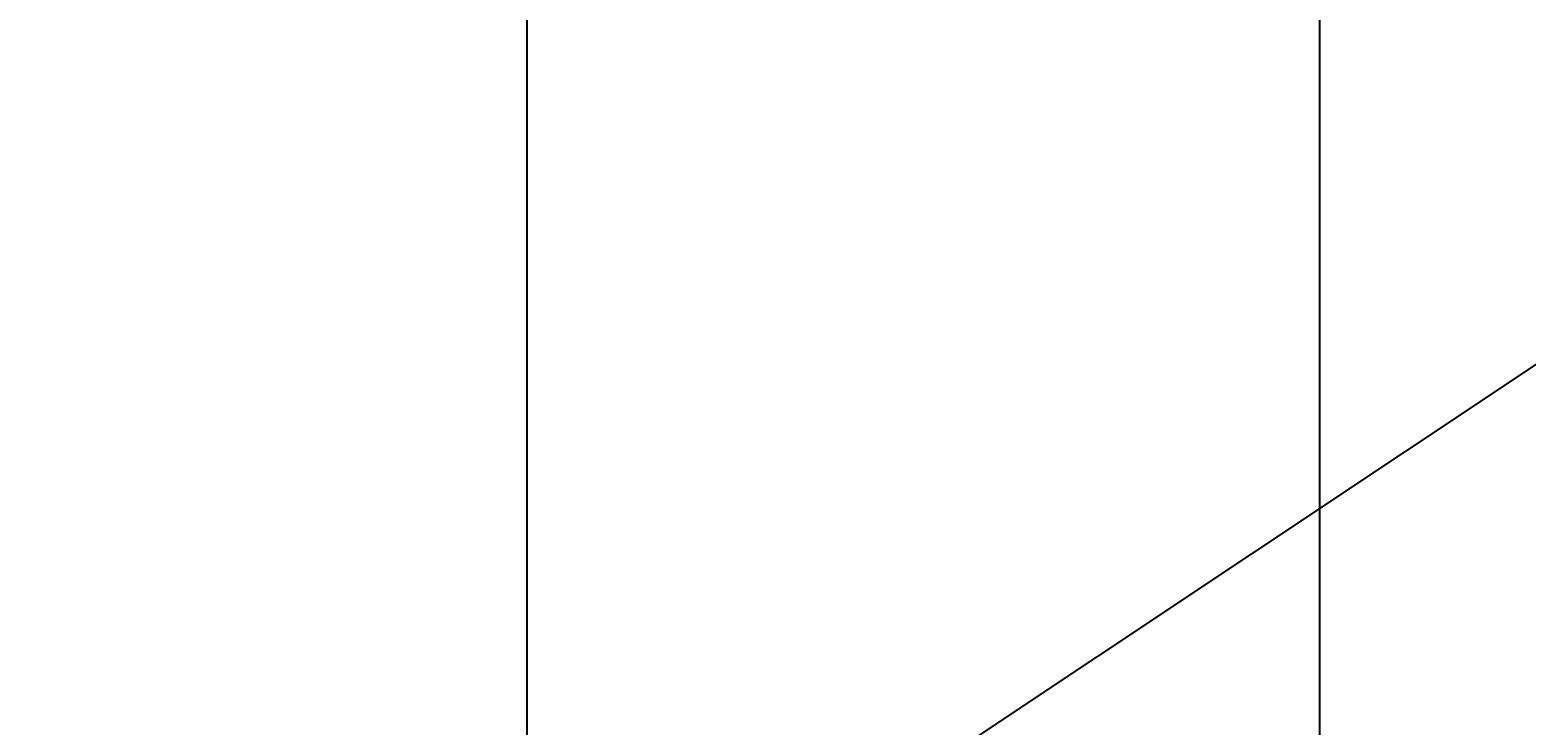
# Model space of a CAD drawing. Units: inches. Extents: x 35362 to 73946, y 43607 to 67532.
# Tile 120 of 134: x 50905 to 51049, y 49128 to 49195. Entities that reach past the tile are written whole.
import ezdxf

# ---------------------------------------------------------------- set-up
doc = ezdxf.new("R2010")
doc.units = ezdxf.units.IN
doc.header["$MEASUREMENT"] = 0
doc.layers.add('A-ANNO-DIMS', color=2, linetype='Continuous', lineweight=18)
doc.layers.add('E-SYMB', color=1, linetype='Continuous', lineweight=25)
doc.styles.get("Standard").update_dxf_attribs({"font": 'arial.ttf'})
doc.dimstyles.get("Standard").update_dxf_attribs({"dimtxt": 0.18, "dimasz": 0.18, "dimexe": 0.18, "dimexo": 0.0625, "dimgap": 0.09, "dimtad": 0, "dimtih": 1, "dimtoh": 1, "dimdec": 4, "dimzin": 0, "dimdsep": 46, "dimtxsty": 'Standard', "dimcen": 0.09, "dimadec": 0, "dimazin": 0, "dimtfac": 1, "dimtdec": 4, "dimtofl": 0, "dimtmove": 0, "dimatfit": 3, "dimfxl": 1, "dimtolj": 1, "dimtzin": 0, "dimarcsym": 0})

# ---------------------------------------------------------------- blocks, each defined once
blk = doc.blocks.new('*D11')
at = {"layer": 'A-ANNO-DIMS', "color": 0, "lineweight": -2, "transparency": 16777216}
for p, q in [((47978.66, 56028.77), (47978.66, 43606.68)), ((53109.76, 56028.77), (53109.76, 43606.68)), ((47978.84, 43606.86), (50543.87, 43606.86)), ((53109.58, 43606.86), (50544.55, 43606.86))]:
    blk.add_line(p, q, dxfattribs=at)
at = {"layer": 'A-ANNO-DIMS', "color": 0, "transparency": 16777216}
for points in [[(47978.84, 43606.89), (47978.84, 43606.83), (47978.66, 43606.86)], [(53109.58, 43606.89), (53109.58, 43606.83), (53109.76, 43606.86)]]:
    blk.add_solid(points, dxfattribs=at)
at = {"layer": 'Defpoints', "color": 0, "transparency": 16777216}
for p in [(47978.66, 56028.84), (53109.76, 56028.84), (53109.76, 43606.86)]:
    blk.add_point(p, dxfattribs=at)
at = {"layer": 'A-ANNO-DIMS', "color": 0, "transparency": 16777216, "insert": (50544.21, 43606.86), "char_height": 0.18, "attachment_point": 5}
blk.add_mtext('\\A1;5131', dxfattribs=at)
blk = doc.blocks.new('*D13')
at = {"layer": 'A-ANNO-DIMS', "color": 0, "lineweight": -2, "transparency": 16777216}
for p, q in [((48373.49, 51694.02), (48373.49, 43606.68)), ((51029.04, 51694.02), (51029.04, 43606.68)), ((48373.67, 43606.86), (49700.8, 43606.86)), ((51028.86, 43606.86), (49701.73, 43606.86))]:
    blk.add_line(p, q, dxfattribs=at)
at = {"layer": 'A-ANNO-DIMS', "color": 0, "transparency": 16777216}
for points in [[(48373.67, 43606.89), (48373.67, 43606.83), (48373.49, 43606.86)], [(51028.86, 43606.89), (51028.86, 43606.83), (51029.04, 43606.86)]]:
    blk.add_solid(points, dxfattribs=at)
at = {"layer": 'Defpoints', "color": 0, "transparency": 16777216}
for p in [(48373.49, 51694.09), (51029.04, 51694.09), (51029.04, 43606.86)]:
    blk.add_point(p, dxfattribs=at)
at = {"layer": 'A-ANNO-DIMS', "color": 0, "transparency": 16777216, "insert": (49701.27, 43606.86), "char_height": 0.18, "attachment_point": 5}
blk.add_mtext('\\A1;2655.6', dxfattribs=at)
blk = doc.blocks.new('*D17')
at = {"layer": 'A-ANNO-DIMS', "color": 0, "lineweight": -2, "transparency": 16777216}
for p, q in [((49923.31, 61293.22), (49923.31, 43606.68)), ((51913.93, 61293.22), (51913.93, 43606.68)), ((49923.49, 43606.86), (50918.16, 43606.86)), ((51913.75, 43606.86), (50919.07, 43606.86))]:
    blk.add_line(p, q, dxfattribs=at)
at = {"layer": 'A-ANNO-DIMS', "color": 0, "transparency": 16777216}
for points in [[(49923.49, 43606.89), (49923.49, 43606.83), (49923.31, 43606.86)], [(51913.75, 43606.89), (51913.75, 43606.83), (51913.93, 43606.86)]]:
    blk.add_solid(points, dxfattribs=at)
at = {"layer": 'Defpoints', "color": 0, "transparency": 16777216}
for p in [(49923.31, 61293.29), (51913.93, 61293.29), (51913.93, 43606.86)]:
    blk.add_point(p, dxfattribs=at)
at = {"layer": 'A-ANNO-DIMS', "color": 0, "transparency": 16777216, "insert": (50918.62, 43606.86), "char_height": 0.18, "attachment_point": 5}
blk.add_mtext('\\A1;1990.6', dxfattribs=at)
blk = doc.blocks.new('*D67')
at = {"layer": 'A-ANNO-DIMS', "color": 0, "lineweight": -2, "transparency": 16777216}
for p, q in [((56873.54, 53351.53), (35361.77, 53351.53)), ((35361.95, 53351.35), (35361.95, 49400.89)), ((35361.95, 45450.07), (35361.95, 49400.53)), ((53793.58, 45449.89), (35361.77, 45449.89))]:
    blk.add_line(p, q, dxfattribs=at)
at = {"layer": 'A-ANNO-DIMS', "color": 0, "transparency": 16777216}
for points in [[(35361.92, 53351.35), (35361.98, 53351.35), (35361.95, 53351.53)], [(35361.92, 45450.07), (35361.98, 45450.07), (35361.95, 45449.89)]]:
    blk.add_solid(points, dxfattribs=at)
at = {"layer": 'Defpoints', "color": 0, "transparency": 16777216}
for p in [(35361.95, 53351.53), (56873.6, 53351.53), (53793.64, 45449.89)]:
    blk.add_point(p, dxfattribs=at)
at = {"layer": 'A-ANNO-DIMS', "color": 0, "transparency": 16777216, "insert": (35361.95, 49400.71), "char_height": 0.18, "attachment_point": 5}
blk.add_mtext('\\A1;7901.6', dxfattribs=at)
blk = doc.blocks.new('*D84')
at = {"layer": 'A-ANNO-DIMS', "color": 0, "lineweight": -2, "transparency": 16777216}
for p, q in [((55540.23, 49259.94), (35361.77, 49259.94)), ((35361.95, 49259.76), (35361.95, 49115.14)), ((35361.95, 48970.16), (35361.95, 49114.78)), ((55540.23, 48969.98), (35361.77, 48969.98))]:
    blk.add_line(p, q, dxfattribs=at)
at = {"layer": 'A-ANNO-DIMS', "color": 0, "transparency": 16777216}
for points in [[(35361.92, 49259.76), (35361.98, 49259.76), (35361.95, 49259.94)], [(35361.92, 48970.16), (35361.98, 48970.16), (35361.95, 48969.98)]]:
    blk.add_solid(points, dxfattribs=at)
at = {"layer": 'Defpoints', "color": 0, "transparency": 16777216}
for p in [(35361.95, 49259.94), (55540.3, 49259.94), (55540.3, 48969.98)]:
    blk.add_point(p, dxfattribs=at)
at = {"layer": 'A-ANNO-DIMS', "color": 0, "transparency": 16777216, "insert": (35361.95, 49114.96), "char_height": 0.18, "attachment_point": 5}
blk.add_mtext('\\A1;289.96', dxfattribs=at)
blk = doc.blocks.new('*D85')
at = {"layer": 'A-ANNO-DIMS', "color": 0, "lineweight": -2, "transparency": 16777216}
for p, q in [((50952.66, 49098.43), (50952.66, 67531.69)), ((51285.59, 49320.14), (51285.59, 67531.69)), ((50952.84, 67531.51), (51118.73, 67531.51)), ((51285.41, 67531.51), (51119.52, 67531.51))]:
    blk.add_line(p, q, dxfattribs=at)
at = {"layer": 'A-ANNO-DIMS', "color": 0, "transparency": 16777216}
for points in [[(50952.84, 67531.54), (50952.84, 67531.48), (50952.66, 67531.51)], [(51285.41, 67531.54), (51285.41, 67531.48), (51285.59, 67531.51)]]:
    blk.add_solid(points, dxfattribs=at)
at = {"layer": 'Defpoints', "color": 0, "transparency": 16777216}
for p in [(51285.59, 67531.51), (51285.59, 49320.08), (50952.66, 49098.37)]:
    blk.add_point(p, dxfattribs=at)
at = {"layer": 'A-ANNO-DIMS', "color": 0, "transparency": 16777216, "insert": (51119.13, 67531.51), "char_height": 0.18, "attachment_point": 5}
blk.add_mtext('\\A1;332.9', dxfattribs=at)
blk = doc.blocks.new('*D86')
at = {"layer": 'A-ANNO-DIMS', "color": 0, "lineweight": -2, "transparency": 16777216}
for p, q in [((51285.53, 49320.08), (35361.77, 49320.08)), ((35361.95, 49319.9), (35361.95, 49120.26)), ((35361.95, 48920.26), (35361.95, 49119.9)), ((51285.53, 48920.08), (35361.77, 48920.08))]:
    blk.add_line(p, q, dxfattribs=at)
at = {"layer": 'A-ANNO-DIMS', "color": 0, "transparency": 16777216}
for points in [[(35361.92, 49319.9), (35361.98, 49319.9), (35361.95, 49320.08)], [(35361.92, 48920.26), (35361.98, 48920.26), (35361.95, 48920.08)]]:
    blk.add_solid(points, dxfattribs=at)
at = {"layer": 'Defpoints', "color": 0, "transparency": 16777216}
for p in [(35361.95, 49320.08), (51285.59, 49320.08), (51285.59, 48920.08)]:
    blk.add_point(p, dxfattribs=at)
at = {"layer": 'A-ANNO-DIMS', "color": 0, "transparency": 16777216, "insert": (35361.95, 49120.08), "char_height": 0.18, "attachment_point": 5}
blk.add_mtext('\\A1;400.0', dxfattribs=at)
blk = doc.blocks.new('*D107')
at = {"layer": 'A-ANNO-DIMS', "color": 0, "lineweight": -2, "transparency": 16777216}
for p, q in [((50139.56, 59850.01), (50139.56, 43606.68)), ((51320.81, 59850.01), (51320.81, 43606.68)), ((50139.74, 43606.86), (50729.73, 43606.86)), ((51320.63, 43606.86), (50730.64, 43606.86))]:
    blk.add_line(p, q, dxfattribs=at)
at = {"layer": 'A-ANNO-DIMS', "color": 0, "transparency": 16777216}
for points in [[(50139.74, 43606.89), (50139.74, 43606.83), (50139.56, 43606.86)], [(51320.63, 43606.89), (51320.63, 43606.83), (51320.81, 43606.86)]]:
    blk.add_solid(points, dxfattribs=at)
at = {"layer": 'Defpoints', "color": 0, "transparency": 16777216}
for p in [(50139.56, 59850.08), (51320.81, 59850.08), (51320.81, 43606.86)]:
    blk.add_point(p, dxfattribs=at)
at = {"layer": 'A-ANNO-DIMS', "color": 0, "transparency": 16777216, "insert": (50730.19, 43606.86), "char_height": 0.18, "attachment_point": 5}
blk.add_mtext('\\A1;1181.3', dxfattribs=at)

msp = doc.modelspace()

# ---------------------------------------------------------------- linework, layer by layer
at = {"layer": 'E-SYMB'}
msp.add_line((51285.595, 49320.079), (50952.662, 49098.368), dxfattribs=at)

# ---------------------------------------------------------------- dimensions: what is measured, and where the dimension line sits
at = {"layer": 'A-ANNO-DIMS'}
for base, p1, p2, override, picture, middle in [((51285.595, 67531.512), (50952.662, 49098.368), (51285.595, 49320.079), {"dimdec": 1, "dimlfac": 1, "dimrnd": 0, "dimzin": 0, "dimdsep": 46, "dimlunit": 2}, '*D85', (51119.128, 67531.512)), ((51913.931, 43606.859), (49923.307, 61293.286), (51913.931, 61293.286), {"dimdec": 1, "dimlfac": 1, "dimrnd": 0, "dimzin": 0, "dimdsep": 46, "dimlunit": 2}, '*D17', (50918.619, 43606.859)), ((51320.8133, 43606.859), (50139.5627, 59850.0769), (51320.8133, 59850.0769), {"dimdec": 1, "dimlfac": 1, "dimrnd": 0, "dimzin": 0, "dimdsep": 46, "dimlunit": 2}, '*D107', (50730.188, 43606.859)), ((53109.76, 43606.859), (47978.665, 56028.836), (53109.76, 56028.836), {"dimdec": 0, "dimlfac": 1, "dimrnd": 0, "dimzin": 0, "dimdsep": 46, "dimlunit": 2}, '*D11', (50544.212, 43606.859)), ((51029.043, 43606.859), (48373.492, 51694.087), (51029.043, 51694.087), {"dimdec": 1, "dimlfac": 1, "dimrnd": 0, "dimzin": 0, "dimdsep": 46, "dimlunit": 2}, '*D13', (49701.267, 43606.859))]:
    dim = msp.add_linear_dim(base=base, p1=p1, p2=p2, dimstyle='Standard', override=override, dxfattribs=at)
    dim.commit()
    dim.dimension.update_dxf_attribs({"geometry": picture, "text_midpoint": middle})
for base, p1, p2, override, picture, middle in [((35361.949, 53351.529), (53793.638, 45449.894), (56873.602, 53351.529), {"dimdec": 1, "dimlfac": 1, "dimrnd": 0, "dimzin": 0, "dimdsep": 46, "dimlunit": 2}, '*D67', (35361.949, 49400.712)), ((35361.949, 49320.079), (51285.595, 48920.079), (51285.595, 49320.079), {"dimdec": 1, "dimlfac": 1, "dimrnd": 0, "dimzin": 0, "dimdsep": 46, "dimlunit": 2}, '*D86', (35361.949, 49120.079)), ((35361.9491, 49259.9353), (55540.2972, 48969.9796), (55540.2972, 49259.9353), {"dimdec": 2, "dimlfac": 1, "dimrnd": 0, "dimzin": 0, "dimdsep": 46, "dimlunit": 2}, '*D84', (35361.9491, 49114.9575))]:
    dim = msp.add_linear_dim(base=base, p1=p1, p2=p2, angle=90, dimstyle='Standard', override=override, dxfattribs=at)
    dim.commit()
    dim.dimension.update_dxf_attribs({"geometry": picture, "text_midpoint": middle})

doc.saveas('drawing.dxf')
